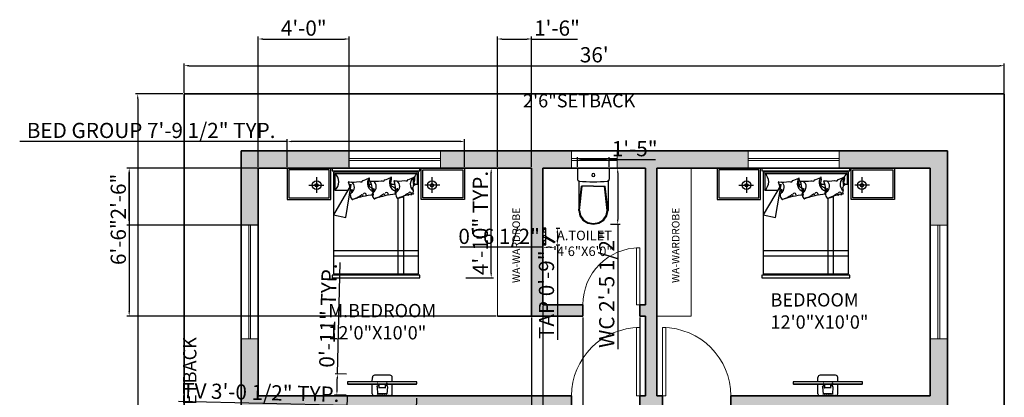
# Model space of a CAD drawing. Units: inches. Extents: x 4732 to 5926, y 2665 to 3255.
# Tile 6 of 8: x 4732 to 5250, y 3056 to 3255. Entities that reach past the tile are written whole.
import ezdxf

# ---------------------------------------------------------------- set-up
doc = ezdxf.new("R2010")
doc.units = ezdxf.units.IN
for name, color, linetype, lineweight in [('A-ANNO-DIMS', 2, 'Continuous', 18), ('A-ANNO-TEXT', 7, 'Continuous', 18), ('A-AREA-IDEN', 7, 'Continuous', 18), ('A-DOOR', 3, 'Continuous', 18), ('A-EQPM', 8, 'Continuous', 18), ('A-FLOR-CASE', 7, 'Continuous', 18), ('A-GLAZ', 4, 'Continuous', 18), ('A-WALL', 7, 'Continuous', 35), ('A-WALL-PATT', 8, 'Continuous', 13), ('C-PROP', 7, 'Continuous', 35), ('NOI THAT', 42, 'Continuous', 18), ('Сантехника', 7, 'Continuous', 18)]:
    doc.layers.add(name, color=color, linetype=linetype, lineweight=lineweight)
for name, color, linetype in [('FUR', 42, 'Continuous'), ('HA', 9, 'Continuous'), ('HID', 11, 'Continuous'), ('SAN', 5, 'Continuous'), ('SANTEH', 7, 'Continuous'), ('window', 130, 'Continuous')]:
    doc.layers.add(name, color=color, linetype=linetype)
doc.styles.get("Standard").update_dxf_attribs({"font": 'arial.ttf'})
doc.dimstyles.new('ISO-25', dxfattribs={"dimtxt": 8, "dimasz": 2.5, "dimexe": 1.25, "dimexo": 0.625, "dimtad": 1, "dimdec": 1, "dimlunit": 3, "dimtxsty": 'Standard', "dimcen": 2.5, "dimadec": 0, "dimazin": 0, "dimtfac": 1, "dimtdec": 1, "dimtmove": 0, "dimatfit": 3, "dimfxl": 1, "dimarcsym": 0})

# ---------------------------------------------------------------- blocks, each defined once
blk = doc.blocks.new('*D1')
at = {"layer": 'A-ANNO-DIMS', "color": 0, "lineweight": -2, "transparency": 16777216}
for p, q in [((4818.38, 3216.56), (4818.38, 3232.07)), ((5250.38, 3216.56), (5250.38, 3232.07)), ((4820.88, 3230.82), (5247.88, 3230.82))]:
    blk.add_line(p, q, dxfattribs=at)
at = {"layer": 'A-ANNO-DIMS', "color": 0, "transparency": 16777216}
for points in [[(4820.88, 3231.24), (4820.88, 3230.41), (4818.38, 3230.82)], [(5247.88, 3231.24), (5247.88, 3230.41), (5250.38, 3230.82)]]:
    blk.add_solid(points, dxfattribs=at)
at = {"layer": 'Defpoints', "color": 0, "transparency": 16777216}
for p in [(5250.38, 3230.82), (4818.38, 3215.93), (5250.38, 3215.93)]:
    blk.add_point(p, dxfattribs=at)
at = {"layer": 'A-ANNO-DIMS', "color": 0, "transparency": 16777216, "insert": (5034.38, 3235.54), "char_height": 8, "attachment_point": 5}
blk.add_mtext("36'", dxfattribs=at)
blk = doc.blocks.new('A$C73A16738')
at = {"layer": 'FUR'}
for p, q in [((1.15, 2.389), (1.1, 2.164)), ((1.7, 2.064), (1.15, 2.389)), ((1.6, 2.364), (1.6, 2.123)), ((1.9, 2.364), (1.6, 2.364)), ((1.9, 2.364), (1.9, 0.864)), ((1.1, 2.164), (1.7, 2.064)), ((1.7, 2.099), (1.7, 2.064)), ((1.7, 1.695), (1.7, 1.735)), ((1.7, 1.268), (1.7, 1.33)), ((1.7, 0.839), (1.7, 0.904)), ((1.9, 0.864), (1.7, 0.864))]:
    blk.add_line(p, q, dxfattribs=at)
for points in [[(1.428, 2.439), (2, 2.439), (2, 3.229), (1.428, 3.229)], [(1.458, 2.469), (1.97, 2.469), (1.97, 3.199), (1.458, 3.199)], [(0, 2.414), (0, 0.814), (0.05, 0.814), (0.05, 2.414)], [(0.075, 0.839), (1.925, 0.839), (1.925, 2.389), (0.075, 2.389)], [(1.95, 2.414), (1.95, 0.814), (2, 0.814), (2, 2.414)], [(1.428, 0.789), (2, 0.789), (2, 0), (1.428, 0)], [(1.458, 0.759), (1.97, 0.759), (1.97, 0.03), (1.458, 0.03)]]:
    blk.add_lwpolyline(points, close=True, dxfattribs=at)
for centre, start, end in [((1.75, 2.481), 217.7826, 322.2174), ((1.75, 0.748), 37.7826, 105.2747)]:
    blk.add_arc(centre, 0.19, start, end, dxfattribs=at)
at = {"layer": 'HA'}
for p, q in [((0.4, 2.389), (0.4, 0.839)), ((0.5, 2.389), (0.5, 0.839)), ((1.446, 1.214), (0.075, 1.214)), ((1.477, 1.114), (0.075, 1.114))]:
    blk.add_line(p, q, dxfattribs=at)
at = {"layer": 'HID'}
for centre, radius, start, end in [((1.442, 2.042), 0.0144, 131.666, 199.4465), ((0.016, 1.539), 1.498, 4.5852, 19.4465), ((0.016, 1.539), 1.498, 16.386, 19.4465), ((1.51, 1.965), 0.117, 87.3377, 131.666), ((1.515, 2.068), 0.0144, 51.6071, 87.3377), ((1.617, 2.197), 0.15, 231.6071, 269.7845), ((1.65, 2.128), 0.12, 212.7628, 323.8922), ((1.592, 2.074), 0.0072, 92.7363, 208.2985), ((1.628, 2.093), 0.0475, 208.2985, 255.7891), ((1.569, 2.56), 0.48, 272.7363, 290.959), ((1.743, 2.106), 0.0072, 352.7248, 110.959), ((2.348, 2.029), 0.603, 172.7248, 190.2702), ((1.467, 1.966), 0.0144, 196.386, 223.7955), ((0.926, 1.551), 0.667, 29.049, 37.3823), ((1.51, 1.823), 0.0319, 112.7015, 147.1556), ((1.51, 1.821), 0.0305, 232.3565, 65.7762), ((1.503, 1.839), 0.0144, 102.6426, 112.7015), ((1.497, 1.868), 0.0144, 282.6426, 29.049), ((2.038, 1.868), 0.288, 169.4168, 179.3085), ((1.758, 1.872), 0.0072, 179.3085, 290.689), ((1.763, 1.858), 0.0072, 16.2196, 110.689), ((2.348, 2.029), 0.603, 196.2196, 208.2114), ((1.455, 1.642), 0.0144, 131.666, 199.4465), ((0.03, 1.139), 1.498, 4.5852, 19.4465), ((0.03, 1.139), 1.498, 16.386, 19.4465), ((1.524, 1.565), 0.117, 87.3377, 131.666), ((1.524, 1.653), 0.0144, 67.1663, 184.3422), ((1.529, 1.668), 0.0144, 51.6071, 87.3377), ((1.574, 1.774), 0.117, 247.1663, 295.7613), ((1.631, 1.797), 0.15, 231.6071, 269.7845), ((1.663, 1.728), 0.12, 212.7628, 323.8922), ((1.722, 1.609), 0.162, 53.8947, 162.3952), ((1.606, 1.674), 0.0072, 92.7363, 208.2985), ((1.642, 1.693), 0.0475, 208.2985, 255.7891), ((1.583, 2.161), 0.48, 272.7363, 290.959), ((2.854, 0.961), 1.418, 145.8329, 150.0245), ((3.143, 2.369), 1.611, 202.7018, 202.7206), ((1.683, 1.758), 0.0288, 232.662, 339.1573), ((1.686, 1.753), 0.0072, 38.8315, 145.8329), ((1.788, 1.924), 0.192, 239.9211, 277.124), ((0.088, 1.831), 1.611, 356.4982, 357.2888), ((1.757, 1.706), 0.0072, 352.7248, 110.959), ((2.362, 1.629), 0.603, 172.7248, 190.2702), ((1.811, 1.74), 0.0072, 277.124, 28.2114), ((1.811, 1.74), 0.0072, 277.124, 28.2114), ((1.48, 1.566), 0.0144, 196.386, 223.7955), ((0.94, 1.151), 0.667, 29.049, 37.3823), ((1.523, 1.423), 0.0319, 112.7015, 147.1556), ((1.523, 1.422), 0.0305, 232.3565, 65.7762), ((1.517, 1.44), 0.0144, 102.6426, 112.7015), ((1.51, 1.468), 0.0144, 282.6426, 29.049), ((2.052, 1.468), 0.288, 169.4168, 179.3085), ((1.771, 1.472), 0.0072, 179.3085, 290.689), ((1.776, 1.458), 0.0072, 16.2196, 110.689), ((2.362, 1.629), 0.603, 196.2196, 208.2114), ((1.529, 1.139), 0.117, 87.3377, 131.666), ((1.537, 1.254), 0.0144, 67.1663, 184.3422), ((1.533, 1.242), 0.0144, 51.6071, 87.3377), ((1.588, 1.374), 0.117, 247.1663, 295.7613), ((1.736, 1.209), 0.162, 53.8947, 162.3952), ((1.611, 1.248), 0.0072, 92.7363, 208.2985), ((1.588, 1.734), 0.48, 272.7363, 290.959), ((2.867, 0.561), 1.418, 145.8329, 150.0245), ((3.156, 1.97), 1.611, 202.7018, 202.7206), ((1.697, 1.359), 0.0288, 232.662, 339.1573), ((1.7, 1.353), 0.0072, 38.8315, 145.8329), ((1.802, 1.524), 0.192, 239.9211, 277.124), ((0.102, 1.431), 1.611, 356.4982, 357.2888), ((1.762, 1.28), 0.0072, 352.7248, 110.959), ((2.367, 1.203), 0.603, 172.7248, 190.2702), ((1.825, 1.34), 0.0072, 277.124, 28.2114), ((1.825, 1.34), 0.0072, 277.124, 28.2114), ((1.46, 1.216), 0.0144, 131.666, 199.4465), ((0.688, 0.841), 0.844, 6.224, 26.0326), ((0.034, 0.713), 1.498, 16.386, 19.4465), ((1.485, 1.14), 0.0144, 196.386, 223.7955), ((0.945, 0.725), 0.667, 29.049, 37.3823), ((1.635, 1.371), 0.15, 231.6071, 269.7845), ((1.668, 1.302), 0.12, 212.7628, 323.8922), ((1.646, 1.267), 0.0475, 208.2985, 255.7891), ((2.056, 1.042), 0.288, 169.4168, 179.3085), ((1.528, 0.997), 0.0319, 112.7015, 147.1556), ((1.528, 0.995), 0.0305, 232.3565, 65.7762), ((1.521, 1.013), 0.0144, 102.6426, 112.7015), ((1.515, 1.042), 0.0144, 282.6426, 29.049), ((1.542, 0.927), 0.0144, 67.1663, 184.3422), ((1.593, 1.048), 0.117, 247.1663, 295.7613), ((1.705, 0.84), 0.15, 29.3598, 142.4281), ((1.581, 0.528), 0.419, 73.7524, 81.4605), ((3.161, 1.543), 1.611, 202.7018, 202.7206), ((1.702, 0.932), 0.0288, 232.662, 339.1573), ((1.705, 0.927), 0.0072, 38.8315, 145.8329), ((0.106, 1.005), 1.611, 356.4982, 357.2888), ((1.806, 1.098), 0.192, 246.1093, 277.124), ((1.776, 1.046), 0.0072, 179.3085, 290.689), ((1.781, 1.032), 0.0072, 16.2196, 110.689), ((2.367, 1.203), 0.603, 196.2196, 208.2114), ((1.829, 0.914), 0.0072, 277.124, 28.2114), ((1.829, 0.914), 0.0072, 277.124, 28.2114)]:
    blk.add_arc(centre, radius, start, end, dxfattribs=at)
at = {"layer": 'SAN'}
for p, q in [((1.832, 2.695), (1.546, 2.695)), ((1.688, 2.835), (1.688, 2.566)), ((1.688, 0.454), (1.688, 0.723)), ((1.832, 0.594), (1.546, 0.594))]:
    blk.add_line(p, q, dxfattribs=at)
for centre, radius in [((1.688, 2.695), 0.08), ((1.688, 2.695), 0.03), ((1.688, 0.594), 0.08), ((1.688, 0.594), 0.03)]:
    blk.add_circle(centre, radius, dxfattribs=at)
blk = doc.blocks.new('*U19')
for p, q in [((0, 0), (0, -6)), ((30, 0), (30, -6))]:
    blk.add_line(p, q)
blk.add_lwpolyline([(0, 0), (0, 30), (1.75, 30), (1.75, 0)], close=True)
blk.add_arc((0, 0), 30, 0, 90)
blk = doc.blocks.new('*U20')
for p, q in [((0, 0), (0, -6)), ((36, 0), (36, -6))]:
    blk.add_line(p, q)
blk.add_lwpolyline([(0, 0), (0, 36), (1.75, 36), (1.75, 0)], close=True)
blk.add_arc((0, 0), 36, 0, 90)
blk = doc.blocks.new('WC 2 Symb_109')
at = {"layer": 'SANTEH'}
for p, q in [((0, 0), (0, 380)), ((0, 380), (132, 380)), ((154, 365), (507, 365)), ((506, 365), (216, 331)), ((506, 356), (216, 322)), ((216, 190), (216, 331)), ((216, 190), (216, 49)), ((154, 15), (507, 15)), ((506, 24), (216, 58)), ((506, 15), (216, 49)), ((0, 0), (132, 0))]:
    blk.add_line(p, q, dxfattribs=at)
for points in [[(155, 360), (154, 364), (152, 368), (150, 371), (147, 374), (144, 377), (140, 379), (137, 380), (132, 380)], [(155, 20), (159, 62), (161, 105), (163, 147), (164, 190), (163, 233), (161, 275), (159, 318), (155, 360)], [(506, 24), (565, 37), (616, 73), (649, 126), (661, 190), (649, 254), (616, 307), (565, 343), (506, 356)], [(507, 15), (569, 28), (622, 66), (658, 123), (670, 190), (658, 257), (622, 314), (569, 352), (507, 365)], [(132, 0), (136, 0), (140, 1), (144, 3), (147, 6), (150, 9), (152, 12), (154, 16), (155, 20)]]:
    blk.add_lwpolyline(points, dxfattribs=at)
blk.add_lwpolyline([(84, 208), (70, 203), (65, 190), (70, 177), (84, 172), (97, 177), (102, 190), (97, 203)], close=True, dxfattribs=at)
blk = doc.blocks.new('Faucet - kit sink top')
at = {"layer": 'SANTEH'}
for p, q in [((-5.5, -0.75), (-5.5, -1.25)), ((-4.94278, -0.75), (-5.5, -0.75)), ((-5.5, -1.25), (-4.94278, -1.25)), ((-0.14775, -1.7441), (3.56698, -8.1782)), ((4.43301, -7.6782), (0.71828, -1.2441)), ((4.94278, -0.75), (5.5, -0.75)), ((5.5, -1.25), (4.94278, -1.25)), ((5.5, -0.75), (5.5, -1.25))]:
    blk.add_line(p, q, dxfattribs=at)
blk.add_lwpolyline([(-0.00587, -2), (-6, -2), (-6, 0), (6, 0), (6, -2), (1.15195, -2)], dxfattribs=at)
for centre, radius in [((-4, -1), 1), ((4, -1), 1), ((0, -1), 0.75)]:
    blk.add_circle(centre, radius, dxfattribs=at)
blk.add_arc((4, -7.9282), 0.5, 210, 30, dxfattribs=at)
blk = doc.blocks.new('TV')
at = {"color": 0}
for p, q in [((3967.27, 1784.85), (3967.05, 1784.65)), ((3967.76, 1763.68), (3967.54, 1763.86))]:
    blk.add_line(p, q, dxfattribs=at)
at = {"layer": 'window'}
for p, q in [((3967.54, 1763.86), (3967.05, 1784.65)), ((3966.53, 1775.82), (3964.33, 1775.61)), ((3964.34, 1775.34), (3964.45, 1775.34)), ((3964.34, 1775.31), (3964.43, 1775.32)), ((3964.41, 1777.23), (3967.22, 1777.3)), ((3966.14, 1775.2), (3967.01, 1775.22)), ((3966.14, 1775.18), (3967.27, 1775.2)), ((3966.14, 1775.18), (3966.14, 1775.2)), ((3966.3, 1773.29), (3966.26, 1775.18)), ((3968.01, 1777.32), (3969.36, 1777.35)), ((3964.39, 1773.06), (3964.48, 1773.06)), ((3964.39, 1773.04), (3964.5, 1773.04)), ((3966.61, 1772.66), (3964.4, 1772.77)), ((3966.19, 1773.28), (3967.31, 1773.31)), ((3966.19, 1773.26), (3967.05, 1773.28)), ((3966.19, 1773.26), (3966.19, 1773.28)), ((3964.55, 1771.15), (3967.36, 1771.22)), ((3968.15, 1771.24), (3969.5, 1771.27))]:
    blk.add_line(p, q, dxfattribs=at)
for points in [[(3968.33, 1763.69), (3967.83, 1784.86), (3967.27, 1784.85), (3967.76, 1763.68), (3968.33, 1763.69)], [(3963.86, 1771.81), (3963.75, 1776.54)], [(3964.4, 1772.77), (3964.33, 1775.61)], [(3964.48, 1773.06), (3964.43, 1775.32)], [(3964.5, 1773.04), (3964.45, 1775.34)], [(3970.16, 1771.96), (3970.05, 1776.69)]]:
    blk.add_lwpolyline(points, dxfattribs=at)
for points in [[(3966.53, 1775.82, -0.263666), (3966.93, 1775.69), (3967, 1775.57), (3967.01, 1775.22)], [(3966.61, 1772.66, 0.263666), (3967, 1772.81), (3967.06, 1772.93), (3967.05, 1773.28)]]:
    blk.add_lwpolyline(points, format="xyb", dxfattribs=at)
for centre, radius in [((3963.91, 1775.73), 0.0679), ((3963.93, 1775.17), 0.0679), ((3963.94, 1774.6), 0.0679), ((3967.77, 1775.68), 0.0451), ((3963.95, 1774.04), 0.0679), ((3963.97, 1773.48), 0.0679), ((3963.98, 1772.92), 0.0679), ((3963.99, 1772.35), 0.0679), ((3964.01, 1771.79), 0.0679), ((3967.83, 1772.86), 0.0451)]:
    blk.add_circle(centre, radius, dxfattribs=at)
for centre, start, end in [((3964.42, 1776.56), 91.3414, 181.3414), ((3969.38, 1776.67), 1.3414, 91.3414), ((3964.53, 1771.83), 181.3414, 271.3414), ((3969.49, 1771.94), 271.3414, 1.3414)]:
    blk.add_arc(centre, 0.676, start, end, dxfattribs=at)
blk = doc.blocks.new('*D28')
at = {"layer": 'A-ANNO-DIMS', "color": 0, "lineweight": -2, "transparency": 16777216}
for p, q in [((4817.76, 3215.93), (4792.67, 3215.93)), ((4793.92, 3213.43), (4793.92, 2738.43)), ((4817.76, 2735.93), (4792.67, 2735.93))]:
    blk.add_line(p, q, dxfattribs=at)
at = {"layer": 'A-ANNO-DIMS', "color": 0, "transparency": 16777216}
for points in [[(4793.5, 3213.43), (4794.33, 3213.43), (4793.92, 3215.93)], [(4793.5, 2738.43), (4794.33, 2738.43), (4793.92, 2735.93)]]:
    blk.add_solid(points, dxfattribs=at)
at = {"layer": 'Defpoints', "color": 0, "transparency": 16777216}
for p in [(4818.38, 3215.93), (4793.92, 2735.93), (4818.38, 2735.93)]:
    blk.add_point(p, dxfattribs=at)
at = {"layer": 'A-ANNO-DIMS', "color": 0, "transparency": 16777216, "insert": (4789.21, 2975.93), "char_height": 8, "attachment_point": 5, "rotation": 90}
blk.add_mtext("40'", dxfattribs=at)
blk = doc.blocks.new('GLAZ-UNIT-48IN')
for p, q in [((0, 1), (48, 1)), ((0, 0), (48, 0))]:
    blk.add_line(p, q)
blk = doc.blocks.new('GLAZ-UNIT-60IN')
for p, q in [((0, 0), (0, 60)), ((1, 0), (1, 60))]:
    blk.add_line(p, q)
blk = doc.blocks.new('GLAZ-UNIT-24IN')
for p, q in [((0, 1), (24, 1)), ((0, 0), (24, 0))]:
    blk.add_line(p, q)
blk = doc.blocks.new('*D74')
at = {"layer": 'A-ANNO-DIMS', "color": 0, "lineweight": -2, "transparency": 16777216}
for p, q in [((4872.72, 3190.94), (4731.74, 3190.94)), ((4872.72, 3177.56), (4872.72, 3192.19)), ((4963.6, 3190.94), (4875.22, 3190.94)), ((4966.1, 3177.56), (4966.1, 3192.19))]:
    blk.add_line(p, q, dxfattribs=at)
at = {"layer": 'A-ANNO-DIMS', "color": 0, "transparency": 16777216}
for points in [[(4875.22, 3191.36), (4875.22, 3190.52), (4872.72, 3190.94)], [(4963.6, 3191.36), (4963.6, 3190.52), (4966.1, 3190.94)]]:
    blk.add_solid(points, dxfattribs=at)
at = {"layer": 'Defpoints', "color": 0, "transparency": 16777216}
for p in [(4872.72, 3190.94), (4872.72, 3176.93), (4966.1, 3176.93)]:
    blk.add_point(p, dxfattribs=at)
at = {"layer": 'A-ANNO-DIMS', "color": 0, "transparency": 16777216, "insert": (4800.98, 3195.7), "char_height": 8, "attachment_point": 5, "rotation": 360}
blk.add_mtext('BED GROUP 7\'-9 1/2" TYP.', dxfattribs=at)
blk = doc.blocks.new('*D75')
at = {"layer": 'A-ANNO-DIMS', "color": 0, "lineweight": -2, "transparency": 16777216}
for p, q in [((4966.72, 3176.93), (4981.35, 3176.93)), ((4980.1, 3121.59), (4980.1, 3174.43)), ((4966.72, 3119.09), (4981.35, 3119.09))]:
    blk.add_line(p, q, dxfattribs=at)
at = {"layer": 'A-ANNO-DIMS', "color": 0, "transparency": 16777216}
for points in [[(4979.69, 3174.43), (4980.52, 3174.43), (4980.1, 3176.93)], [(4979.69, 3121.59), (4980.52, 3121.59), (4980.1, 3119.09)]]:
    blk.add_solid(points, dxfattribs=at)
at = {"layer": 'Defpoints', "color": 0, "transparency": 16777216}
for p in [(4966.1, 3176.93), (4980.1, 3176.93), (4966.1, 3119.09)]:
    blk.add_point(p, dxfattribs=at)
at = {"layer": 'A-ANNO-DIMS', "color": 0, "transparency": 16777216, "insert": (4975.4, 3148.01), "char_height": 8, "attachment_point": 5, "rotation": 90}
blk.add_mtext('4\'-10" TYP.', dxfattribs=at)
blk = doc.blocks.new('*D82')
at = {"layer": 'A-ANNO-DIMS', "color": 0, "lineweight": -2, "transparency": 16777216}
for p, q in [((4904.29, 3056.7), (4904.13, 3050.59)), ((4940.81, 3055.77), (4940.65, 3049.66)), ((4904.16, 3051.84), (4815.45, 3054.1)), ((4938.19, 3050.98), (4906.66, 3051.78))]:
    blk.add_line(p, q, dxfattribs=at)
at = {"layer": 'A-ANNO-DIMS', "color": 0, "transparency": 16777216}
for points in [[(4906.67, 3052.2), (4906.65, 3051.36), (4904.16, 3051.84)], [(4938.2, 3051.39), (4938.17, 3050.56), (4940.68, 3050.91)]]:
    blk.add_solid(points, dxfattribs=at)
at = {"layer": 'Defpoints', "color": 0, "transparency": 16777216}
for p in [(4904.3, 3057.32), (4940.82, 3056.39), (4904.16, 3051.84)]:
    blk.add_point(p, dxfattribs=at)
at = {"layer": 'A-ANNO-DIMS', "color": 0, "transparency": 16777216, "insert": (4858.68, 3057.76), "char_height": 8, "attachment_point": 5, "rotation": 358.5431}
blk.add_mtext('TV 3\'-0 1/2" TYP.', dxfattribs=at)
blk = doc.blocks.new('*D83')
at = {"layer": 'A-ANNO-DIMS', "color": 0, "lineweight": -2, "transparency": 16777216}
for p, q in [((4899.11, 3068.54), (4900.6, 3127.25)), ((4903.96, 3068.41), (4897.86, 3068.57)), ((4898.89, 3059.96), (4899.04, 3066.04)), ((4903.68, 3057.34), (4897.58, 3057.49))]:
    blk.add_line(p, q, dxfattribs=at)
at = {"layer": 'A-ANNO-DIMS', "color": 0, "transparency": 16777216}
for points in [[(4898.63, 3066.05), (4899.46, 3066.03), (4899.11, 3068.54)], [(4898.47, 3059.97), (4899.3, 3059.95), (4898.82, 3057.46)]]:
    blk.add_solid(points, dxfattribs=at)
at = {"layer": 'Defpoints', "color": 0, "transparency": 16777216}
for p in [(4899.11, 3068.54), (4904.58, 3068.4), (4904.3, 3057.32)]:
    blk.add_point(p, dxfattribs=at)
at = {"layer": 'A-ANNO-DIMS', "color": 0, "transparency": 16777216, "insert": (4895.18, 3099.26), "char_height": 8, "attachment_point": 5, "rotation": 88.5431}
blk.add_mtext('0\'-11" TYP.', dxfattribs=at)
blk = doc.blocks.new('*D98')
at = {"layer": 'A-ANNO-DIMS', "color": 0, "lineweight": -2, "transparency": 16777216}
for p, q in [((5042.94, 3176.93), (5048, 3176.93)), ((5046.75, 3174.43), (5046.75, 3149.83)), ((5042.94, 3147.33), (5048, 3147.33)), ((5046.75, 3147.33), (5046.75, 3081.62))]:
    blk.add_line(p, q, dxfattribs=at)
at = {"layer": 'A-ANNO-DIMS', "color": 0, "transparency": 16777216}
for points in [[(5046.34, 3174.43), (5047.17, 3174.43), (5046.75, 3176.93)], [(5046.34, 3149.83), (5047.17, 3149.83), (5046.75, 3147.33)]]:
    blk.add_solid(points, dxfattribs=at)
at = {"layer": 'Defpoints', "color": 0, "transparency": 16777216}
for p in [(5042.31, 3176.93), (5042.31, 3147.33), (5046.75, 3147.33)]:
    blk.add_point(p, dxfattribs=at)
at = {"layer": 'A-ANNO-DIMS', "color": 0, "transparency": 16777216, "insert": (5041.99, 3113.22), "char_height": 8, "attachment_point": 5, "rotation": 90}
blk.add_mtext('WC 2\'-5 1/2"', dxfattribs=at)
blk = doc.blocks.new('*D99')
at = {"layer": 'A-ANNO-DIMS', "color": 0, "lineweight": -2, "transparency": 16777216}
for p, q in [((5025.52, 3177.56), (5025.52, 3182.62)), ((5028.02, 3181.37), (5039.81, 3181.37)), ((5042.31, 3177.56), (5042.31, 3182.62)), ((5042.31, 3181.37), (5066.57, 3181.37))]:
    blk.add_line(p, q, dxfattribs=at)
at = {"layer": 'A-ANNO-DIMS', "color": 0, "transparency": 16777216}
for points in [[(5028.02, 3181.79), (5028.02, 3180.96), (5025.52, 3181.37)], [(5039.81, 3181.79), (5039.81, 3180.96), (5042.31, 3181.37)]]:
    blk.add_solid(points, dxfattribs=at)
at = {"layer": 'Defpoints', "color": 0, "transparency": 16777216}
for p in [(5042.31, 3181.37), (5025.52, 3176.93), (5042.31, 3176.93)]:
    blk.add_point(p, dxfattribs=at)
at = {"layer": 'A-ANNO-DIMS', "color": 0, "transparency": 16777216, "insert": (5055.69, 3186.08), "char_height": 8, "attachment_point": 5}
blk.add_mtext('1\'-5"', dxfattribs=at)
blk = doc.blocks.new('*D100')
at = {"layer": 'A-ANNO-DIMS', "color": 0, "lineweight": -2, "transparency": 16777216}
for p, q in [((5014.26, 3145.35), (5016.21, 3145.35)), ((5014.96, 3142.85), (5014.96, 3139.02)), ((5014.26, 3136.52), (5016.21, 3136.52)), ((5014.96, 3136.52), (5014.96, 3086.46))]:
    blk.add_line(p, q, dxfattribs=at)
at = {"layer": 'A-ANNO-DIMS', "color": 0, "transparency": 16777216}
for points in [[(5014.54, 3142.85), (5015.37, 3142.85), (5014.96, 3145.35)], [(5014.54, 3139.02), (5015.37, 3139.02), (5014.96, 3136.52)]]:
    blk.add_solid(points, dxfattribs=at)
at = {"layer": 'Defpoints', "color": 0, "transparency": 16777216}
for p in [(5013.63, 3145.35), (5013.63, 3136.52), (5014.96, 3136.52)]:
    blk.add_point(p, dxfattribs=at)
at = {"layer": 'A-ANNO-DIMS', "color": 0, "transparency": 16777216, "insert": (5010.25, 3110.24), "char_height": 8, "attachment_point": 5, "rotation": 90}
blk.add_mtext('TAP 0\'-9"', dxfattribs=at)
blk = doc.blocks.new('*D101')
at = {"layer": 'A-ANNO-DIMS', "color": 0, "lineweight": -2, "transparency": 16777216}
for p, q in [((5007.38, 3135.2), (4963.72, 3135.2)), ((5007.38, 3135.89), (5007.38, 3133.95)), ((5011.13, 3135.2), (5009.88, 3135.2)), ((5013.63, 3135.89), (5013.63, 3133.95))]:
    blk.add_line(p, q, dxfattribs=at)
at = {"layer": 'A-ANNO-DIMS', "color": 0, "transparency": 16777216}
for points in [[(5009.88, 3135.61), (5009.88, 3134.78), (5007.38, 3135.2)], [(5011.13, 3135.61), (5011.13, 3134.78), (5013.63, 3135.2)]]:
    blk.add_solid(points, dxfattribs=at)
at = {"layer": 'Defpoints', "color": 0, "transparency": 16777216}
for p in [(5007.38, 3136.52), (5007.38, 3135.2), (5013.63, 3136.52)]:
    blk.add_point(p, dxfattribs=at)
at = {"layer": 'A-ANNO-DIMS', "color": 0, "transparency": 16777216, "insert": (4984.3, 3139.96), "char_height": 8, "attachment_point": 5}
blk.add_mtext('0\'-6 1/2"', dxfattribs=at)
blk = doc.blocks.new('*D107')
at = {"layer": 'A-ANNO-DIMS', "color": 0, "lineweight": -2, "transparency": 16777216}
for p, q in [((5028.38, 3098.31), (5028.38, 2665.12)), ((5058.38, 3098.31), (5058.38, 2665.12)), ((5030.88, 2666.37), (5055.88, 2666.37))]:
    blk.add_line(p, q, dxfattribs=at)
at = {"layer": 'A-ANNO-DIMS', "color": 0, "transparency": 16777216}
for points in [[(5030.88, 2666.79), (5030.88, 2665.96), (5028.38, 2666.37)], [(5055.88, 2666.79), (5055.88, 2665.96), (5058.38, 2666.37)]]:
    blk.add_solid(points, dxfattribs=at)
at = {"layer": 'Defpoints', "color": 0, "transparency": 16777216}
for p in [(5028.38, 3098.93), (5058.38, 3098.93), (5058.38, 2666.37)]:
    blk.add_point(p, dxfattribs=at)
at = {"layer": 'A-ANNO-DIMS', "color": 0, "transparency": 16777216, "insert": (5043.38, 2671.08), "char_height": 8, "attachment_point": 5}
blk.add_mtext('2\'-6"', dxfattribs=at)
blk = doc.blocks.new('*D108')
at = {"layer": 'A-ANNO-DIMS', "color": 0, "lineweight": -2, "transparency": 16777216}
for p, q in [((4983.38, 3177.56), (4983.38, 3246.13)), ((4985.88, 3244.88), (4998.88, 3244.88)), ((5001.38, 3177.56), (5001.38, 3246.13)), ((5001.38, 3244.88), (5025.64, 3244.88))]:
    blk.add_line(p, q, dxfattribs=at)
at = {"layer": 'A-ANNO-DIMS', "color": 0, "transparency": 16777216}
for points in [[(4985.88, 3245.3), (4985.88, 3244.47), (4983.38, 3244.88)], [(4998.88, 3245.3), (4998.88, 3244.47), (5001.38, 3244.88)]]:
    blk.add_solid(points, dxfattribs=at)
at = {"layer": 'Defpoints', "color": 0, "transparency": 16777216}
for p in [(5001.38, 3244.88), (4983.38, 3176.93), (5001.38, 3176.93)]:
    blk.add_point(p, dxfattribs=at)
at = {"layer": 'A-ANNO-DIMS', "color": 0, "transparency": 16777216, "insert": (5014.76, 3249.59), "char_height": 8, "attachment_point": 5}
blk.add_mtext('1\'-6"', dxfattribs=at)
blk = doc.blocks.new('*D109')
at = {"layer": 'A-ANNO-DIMS', "color": 0, "lineweight": -2, "transparency": 16777216}
for p, q in [((4982.76, 3176.93), (4788.18, 3176.93)), ((4789.43, 3174.43), (4789.43, 3101.43)), ((4982.76, 3098.93), (4788.18, 3098.93))]:
    blk.add_line(p, q, dxfattribs=at)
at = {"layer": 'A-ANNO-DIMS', "color": 0, "transparency": 16777216}
for points in [[(4789.01, 3174.43), (4789.85, 3174.43), (4789.43, 3176.93)], [(4789.01, 3101.43), (4789.85, 3101.43), (4789.43, 3098.93)]]:
    blk.add_solid(points, dxfattribs=at)
at = {"layer": 'Defpoints', "color": 0, "transparency": 16777216}
for p in [(4983.38, 3176.93), (4789.43, 3098.93), (4983.38, 3098.93)]:
    blk.add_point(p, dxfattribs=at)
at = {"layer": 'A-ANNO-DIMS', "color": 0, "transparency": 16777216, "insert": (4784.72, 3137.93), "char_height": 8, "attachment_point": 5, "rotation": 90}
blk.add_mtext('6\'-6"', dxfattribs=at)
blk = doc.blocks.new('*D114')
at = {"layer": 'A-ANNO-DIMS', "color": 0, "lineweight": -2, "transparency": 16777216}
for p, q in [((5007.38, 3104.31), (5007.38, 2665.12)), ((5001.38, 3098.31), (5001.38, 2665.12)), ((4998.88, 2666.37), (4996.38, 2666.37)), ((5001.38, 2666.37), (5007.38, 2666.37)), ((5009.88, 2666.37), (5034.9, 2666.37))]:
    blk.add_line(p, q, dxfattribs=at)
at = {"layer": 'A-ANNO-DIMS', "color": 0, "transparency": 16777216}
for points in [[(4998.88, 2666.79), (4998.88, 2665.96), (5001.38, 2666.37)], [(5009.88, 2666.79), (5009.88, 2665.96), (5007.38, 2666.37)]]:
    blk.add_solid(points, dxfattribs=at)
at = {"layer": 'Defpoints', "color": 0, "transparency": 16777216}
for p in [(5007.38, 3104.93), (5001.38, 3098.93), (5007.38, 2666.37)]:
    blk.add_point(p, dxfattribs=at)
at = {"layer": 'A-ANNO-DIMS', "color": 0, "transparency": 16777216, "insert": (5023.64, 2671.08), "char_height": 8, "attachment_point": 5}
blk.add_mtext('0\'-6"', dxfattribs=at)
blk = doc.blocks.new('*D115')
at = {"layer": 'A-ANNO-DIMS', "color": 0, "lineweight": -2, "transparency": 16777216}
for p, q in [((4857.38, 3177.56), (4857.38, 3246.13)), ((4859.88, 3244.88), (4902.88, 3244.88)), ((4905.38, 3177.56), (4905.38, 3246.13))]:
    blk.add_line(p, q, dxfattribs=at)
at = {"layer": 'A-ANNO-DIMS', "color": 0, "transparency": 16777216}
for points in [[(4859.88, 3245.3), (4859.88, 3244.47), (4857.38, 3244.88)], [(4902.88, 3245.3), (4902.88, 3244.47), (4905.38, 3244.88)]]:
    blk.add_solid(points, dxfattribs=at)
at = {"layer": 'Defpoints', "color": 0, "transparency": 16777216}
for p in [(4905.38, 3244.88), (4857.38, 3176.93), (4905.38, 3176.93)]:
    blk.add_point(p, dxfattribs=at)
at = {"layer": 'A-ANNO-DIMS', "color": 0, "transparency": 16777216, "insert": (4881.38, 3249.59), "char_height": 8, "attachment_point": 5}
blk.add_mtext('4\'-0"', dxfattribs=at)
blk = doc.blocks.new('*D116')
at = {"layer": 'A-ANNO-DIMS', "color": 0, "lineweight": -2, "transparency": 16777216}
for p, q in [((4856.76, 3176.93), (4788.18, 3176.93)), ((4789.43, 3149.43), (4789.43, 3174.43)), ((4856.76, 3146.93), (4788.18, 3146.93))]:
    blk.add_line(p, q, dxfattribs=at)
at = {"layer": 'A-ANNO-DIMS', "color": 0, "transparency": 16777216}
for points in [[(4789.01, 3174.43), (4789.85, 3174.43), (4789.43, 3176.93)], [(4789.01, 3149.43), (4789.85, 3149.43), (4789.43, 3146.93)]]:
    blk.add_solid(points, dxfattribs=at)
at = {"layer": 'Defpoints', "color": 0, "transparency": 16777216}
for p in [(4789.43, 3176.93), (4857.38, 3176.93), (4857.38, 3146.93)]:
    blk.add_point(p, dxfattribs=at)
at = {"layer": 'A-ANNO-DIMS', "color": 0, "transparency": 16777216, "insert": (4784.72, 3161.93), "char_height": 8, "attachment_point": 5, "rotation": 90}
blk.add_mtext('2\'-6"', dxfattribs=at)

msp = doc.modelspace()

# ---------------------------------------------------------------- hatches: boundary and pattern name
at = {"layer": 'A-WALL-PATT'}
h = msp.add_hatch(color=256, dxfattribs=at)
h.dxf.hatch_style = 1
h.paths.add_polyline_path([(4905.38, 3185.93), (4848.38, 3185.93), (4848.38, 3146.93), (4857.38, 3146.93), (4857.38, 3176.93), (4905.38, 3176.93)])
h.paths.add_polyline_path([(5022.38, 3185.93), (4953.38, 3185.93), (4953.38, 3176.93), (4966.1, 3176.93), (5001.38, 3176.93), (5001.38, 3098.93), (5028.38, 3098.93), (5028.38, 3104.93), (5007.38, 3104.93), (5007.38, 3176.93), (5022.38, 3176.93)])
h.paths.add_polyline_path([(5115.38, 3185.93), (5046.38, 3185.93), (5046.38, 3176.93), (5061.38, 3176.93), (5061.38, 3104.93), (5058.38, 3104.93), (5058.38, 3098.93), (5067.38, 3098.93), (5067.38, 3176.93), (5115.38, 3176.93)])
h.paths.add_polyline_path([(5220.38, 3185.93), (5163.38, 3185.93), (5163.38, 3176.93), (5168.97, 3176.93), (5211.38, 3176.93), (5211.38, 3146.93), (5220.38, 3146.93)])
h.paths.add_polyline_path([(4857.38, 3086.93), (4848.38, 3086.93), (4848.38, 3026.93), (4857.38, 3026.93), (4857.38, 3050.93), (5001.38, 3050.93), (5001.38, 3008.93), (5007.38, 3008.93), (5007.38, 3050.93), (5022.38, 3050.93), (5022.38, 3056.93), (4857.38, 3056.93)])
h.paths.add_polyline_path([(4857.38, 2978.93), (4848.38, 2978.93), (4848.38, 2945.93), (4872.38, 2945.93), (4872.38, 2933.93), (4875.38, 2933.93), (4881.38, 2933.93), (4881.38, 2954.93), (4857.38, 2954.93)])
h.paths.add_polyline_path([(4881.38, 2903.93), (4875.38, 2903.93), (4872.38, 2903.93), (4872.38, 2897.93), (4881.38, 2897.93)])
h.paths.add_polyline_path([(4881.38, 2849.93), (4872.38, 2849.93), (4872.38, 2828.75), (4872.38, 2825.93), (4848.38, 2825.93), (4848.38, 2804.93), (4857.38, 2804.93), (4857.38, 2816.93), (4929.38, 2816.93), (4929.38, 2825.93), (4881.38, 2825.93)])
h.paths.add_polyline_path([(4975.38, 2744.93), (4857.38, 2744.93), (4857.38, 2756.93), (4848.38, 2756.93), (4848.38, 2735.93), (4975.38, 2735.93)])
h.paths.add_polyline_path([(5160.38, 2915.93), (5160.38, 2918.93), (5007.38, 2918.93), (5007.38, 2960.93), (5001.38, 2960.93), (5001.38, 2825.93), (4977.38, 2825.93), (4977.38, 2816.93), (5010.38, 2816.93), (5010.38, 2909.93), (5160.38, 2909.93)])
h.paths.add_polyline_path([(5220.38, 2948.93), (5211.38, 2948.93), (5211.38, 2918.93), (5208.38, 2918.93), (5208.38, 2909.93), (5220.38, 2909.93)])
h.paths.add_polyline_path([(5220.38, 3086.93), (5211.38, 3086.93), (5211.38, 3056.93), (5106.38, 3056.93), (5106.38, 3050.93), (5211.38, 3050.93), (5211.38, 3020.93), (5220.38, 3020.93)])
h.paths.add_polyline_path([(5067.38, 3098.93), (5061.38, 3098.93), (5061.38, 3056.93), (5058.38, 3056.93), (5058.38, 3050.93), (5061.38, 3050.93), (5070.38, 3050.93), (5070.38, 3056.93), (5067.38, 3056.93)])
h.paths.add_polyline_path([(4883.76, 2941.13), (4938.24, 2941.13), (4938.24, 2949.38), (4883.76, 2949.38)], flags=9)
h.paths.add_polyline_path([(4840.48, 3026.79), (4840.48, 3093.88), (4825.54, 3093.88), (4825.54, 3026.79)], flags=9)
h.paths.add_polyline_path([(5245.66, 2994.98), (5245.66, 3062.07), (5230.72, 3062.07), (5230.72, 2994.98)], flags=9)
h.paths.add_polyline_path([(4994.89, 3193.24), (5061.99, 3193.24), (5061.99, 3208.18), (4994.89, 3208.18)], flags=9)
h.paths.add_polyline_path([(5081.53, 3115.35), (5081.53, 3161.13), (5073.28, 3161.13), (5073.28, 3115.35)], flags=25)
h.paths.add_polyline_path([(4997.53, 3115.35), (4997.53, 3161.13), (4989.28, 3161.13), (4989.28, 3115.35)], flags=25)
h.paths.add_polyline_path([(5175.31, 2866.04), (5202.42, 2866.04), (5202.42, 2876.71), (5175.31, 2876.71)], flags=9)
h.paths.add_polyline_path([(4820.13, 2876.28), (4869.1, 2876.28), (4869.1, 2902.89), (4820.13, 2902.89)], flags=9)
h.paths.add_polyline_path([(5104.69, 2868.81), (5158.82, 2868.81), (5158.82, 2895.42), (5104.69, 2895.42)], flags=25)
h.paths.add_polyline_path([(5084.11, 2966.75), (5138.25, 2966.75), (5138.25, 2993.36), (5084.11, 2993.36)], flags=9)
h.paths.add_polyline_path([(4897.84, 3000.24), (4946.81, 3000.24), (4946.81, 3026.85), (4897.84, 3026.85)], flags=9)
h.paths.add_polyline_path([(5009.53, 3133.48), (5059.32, 3133.48), (5059.32, 3160.09), (5009.53, 3160.09)], flags=9)
h.paths.add_polyline_path([(5124.24, 3088.37), (5180.47, 3088.37), (5180.47, 3114.99), (5124.24, 3114.99)], flags=9)
h.paths.add_polyline_path([(4897.52, 3088.37), (4965.52, 3088.37), (4965.52, 3114.99), (4897.52, 3114.99)], flags=9)
h.paths.add_polyline_path([(4924.5, 2879.19), (4978.63, 2879.19), (4978.63, 2905.8), (4924.5, 2905.8)], flags=9)

# ---------------------------------------------------------------- linework, layer by layer
at = {"layer": 'A-FLOR-CASE'}
for p, q in [((4983.38, 3098.93), (4983.38, 3176.93)), ((5085.38, 3176.93), (5085.38, 3098.93)), ((5067.38, 3098.93), (5085.38, 3098.93))]:
    msp.add_line(p, q, dxfattribs=at)
at = {"layer": 'A-GLAZ'}
for p, q in [((4905.38, 3176.93), (4905.38, 3185.93)), ((4953.38, 3176.93), (4953.38, 3185.93)), ((5022.38, 3176.93), (5022.38, 3185.93)), ((5046.38, 3176.93), (5046.38, 3185.93)), ((5115.38, 3176.93), (5115.38, 3185.93)), ((5163.38, 3176.93), (5163.38, 3185.93)), ((4857.38, 3146.93), (4848.38, 3146.93)), ((5211.38, 3146.93), (5220.38, 3146.93)), ((4857.38, 3086.93), (4848.38, 3086.93)), ((5211.38, 3086.93), (5220.38, 3086.93))]:
    msp.add_line(p, q, dxfattribs=at)
at = {"layer": 'A-WALL'}
for p, q in [((4848.38, 3185.93), (5220.38, 3185.93)), ((4848.38, 2945.93), (4848.38, 3185.93)), ((5220.38, 3185.93), (5220.38, 2885.93)), ((4857.38, 3176.93), (5001.38, 3176.93)), ((4857.38, 3056.93), (4857.38, 3176.93)), ((5001.38, 3098.93), (5001.38, 3176.93)), ((5007.38, 3104.93), (5007.38, 3176.93)), ((5007.38, 3176.93), (5061.38, 3176.93)), ((5061.38, 3176.93), (5061.38, 3104.93)), ((5067.38, 3176.93), (5067.38, 3056.93)), ((5067.38, 3176.93), (5211.38, 3176.93)), ((5211.38, 3176.93), (5211.38, 3056.93)), ((5007.38, 3104.93), (5028.38, 3104.93)), ((5028.38, 3104.93), (5028.38, 3098.93)), ((5058.38, 3104.93), (5058.38, 3098.93)), ((5058.38, 3104.93), (5061.38, 3104.93)), ((4983.38, 3098.93), (5028.38, 3098.93)), ((5058.38, 3098.93), (5061.38, 3098.93)), ((5061.38, 3098.93), (5061.38, 3056.93)), ((4857.38, 3056.93), (5022.38, 3056.93)), ((5022.38, 3056.93), (5022.38, 3050.93)), ((5058.38, 3056.93), (5061.38, 3056.93)), ((5058.38, 3056.93), (5058.38, 3050.93)), ((5067.38, 3056.93), (5070.38, 3056.93)), ((5070.38, 3056.93), (5070.38, 3050.93)), ((5106.38, 3056.93), (5106.38, 3050.93)), ((5106.38, 3056.93), (5211.38, 3056.93))]:
    msp.add_line(p, q, dxfattribs=at)
at = {"layer": 'C-PROP'}
msp.add_lwpolyline([(4818.38, 3215.93), (5250.38, 3215.93), (5250.38, 2735.93), (4818.38, 2735.93)], close=True, dxfattribs=at)

# ---------------------------------------------------------------- block references
at = {"layer": 'A-DOOR', "xscale": -1}
for name, p in [('*U19', (5058.38, 3104.93)), ('*U20', (5058.38, 3056.93))]:
    msp.add_blockref(name, p, dxfattribs=at)
at = {"layer": 'A-DOOR'}
msp.add_blockref('*U20', (5070.38, 3056.93), dxfattribs=at)
at = {"layer": 'A-EQPM', "xscale": 1.724488909621177, "yscale": 1.724488909621177, "zscale": 1.724488909621177, "rotation": 88.54308451816136}
for p in [(7807.49, -3854.16), (8042.17, -3854.16)]:
    msp.add_blockref('TV', p, dxfattribs=at)
at = {"layer": 'A-GLAZ'}
for name, p in [('GLAZ-UNIT-48IN', (4905.38, 3180.93)), ('GLAZ-UNIT-24IN', (5022.38, 3180.93)), ('GLAZ-UNIT-48IN', (5115.38, 3180.93)), ('GLAZ-UNIT-60IN', (4852.38, 3086.93))]:
    msp.add_blockref(name, p, dxfattribs=at)
at = {"layer": 'A-GLAZ', "rotation": 180}
msp.add_blockref('GLAZ-UNIT-60IN', (5216.38, 3146.93), dxfattribs=at)
at = {"layer": 'NOI THAT', "xscale": 28.92215291203286, "yscale": 28.92215291203286, "zscale": 28.92215291203286, "rotation": 89.99999999852635}
for p in [(4966.1, 3119.09), (5192.53, 3119.09)]:
    msp.add_blockref('A$C73A16738', p, dxfattribs=at)
at = {"layer": 'Сантехника'}
for name, p, xscale, yscale, zscale, rotation in [('WC 2 Symb_109', (5025.52, 3176.93), 0.0441898926459964, 0.0441898926459964, 0.0441898926459964, 270), ('Faucet - kit sink top', (5007.38, 3140.93), -0.7356136897818673, 0.7356136897818673, 0.7356136897818673, 90)]:
    msp.add_blockref(name, p, dxfattribs=dict(at, xscale=xscale, yscale=yscale, zscale=zscale, rotation=rotation))

# ---------------------------------------------------------------- texts
at = {"layer": 'A-ANNO-TEXT', "insert": (4996.86, 3215.89), "char_height": 7, "attachment_point": 1}
msp.add_mtext_dynamic_manual_height_columns('{\\fTimes New Roman|b0|i0|c0|p18; 2\'6"SETBACK }', width=61.0557, gutter_width=12.5, heights=[0], dxfattribs=at)
at = {"layer": 'A-ANNO-TEXT', "attachment_point": 1, "rotation": 90}
for s, width, insert, char_height in [('WA-WARDROBE', 29.5334, (4991.27, 3116.42), 4), ('WA-WARDROBE', 29.5334, (5075.27, 3116.42), 4), ('{\\fTimes New Roman|b0|i0|c0|p18; 2\'6"SETBACK }', 61.0557, (4817.83, 3028.76), 7)]:
    msp.add_mtext_dynamic_manual_height_columns(s, width=width, gutter_width=12.5, heights=[0], dxfattribs=dict(at, insert=insert, char_height=char_height))
at = {"layer": 'A-AREA-IDEN', "attachment_point": 1}
for s, insert, char_height in [('{\\fTimes New Roman|b0|i0|c0|p18;A.TOILET\\P4\'6"X6\'0"}', (5014.72, 3143.95), 5), ('{\\fTimes New Roman|b0|i0|c0|p18;BEDROOM\\P12\'0"X10\'0"}', (5127.2, 3111.03), 7), ('{\\fTimes New Roman|b0|i0|c0|p18;M.BEDROOM\\P12\'0"X10\'0"}', (4894.3, 3105.37), 7)]:
    msp.add_mtext_dynamic_manual_height_columns(s, width=61.0557, gutter_width=12.5, heights=[0], dxfattribs=dict(at, insert=insert, char_height=char_height))

# ---------------------------------------------------------------- dimensions: what is measured, and where the dimension line sits
at = {"layer": 'A-ANNO-DIMS'}
for base, p1, p2, override, picture, middle in [((4905.38, 3244.88), (4857.38, 3176.93), (4905.38, 3176.93), {"dimdec": 1, "dimlfac": 1, "dimrnd": 0, "dimzin": 1, "dimdsep": 46, "dimlunit": 4, "dimfrac": 2}, '*D115', (4881.38, 3249.59)), ((5001.38, 3244.88), (4983.38, 3176.93), (5001.38, 3176.93), {"dimdec": 1, "dimlfac": 1, "dimrnd": 0, "dimzin": 1, "dimdsep": 46, "dimlunit": 4, "dimfrac": 2}, '*D108', (5014.76, 3249.59)), ((5250.38, 3230.82), (4818.38, 3215.93), (5250.38, 3215.93), {"dimclrd": 0, "dimclre": 0, "dimclrt": 0}, '*D1', (5034.38, 3235.54)), ((5042.31, 3181.37), (5025.52, 3176.93), (5042.31, 3176.93), {"dimdec": 1, "dimlfac": 1, "dimrnd": 0, "dimzin": 1, "dimdsep": 46, "dimlunit": 4, "dimfrac": 2}, '*D99', (5055.69, 3186.08)), ((5007.38, 2666.37), (5001.38, 3098.93), (5007.38, 3104.93), {"dimdec": 1, "dimlfac": 1, "dimrnd": 0, "dimzin": 1, "dimdsep": 46, "dimlunit": 4, "dimfrac": 2}, '*D114', (5023.64, 2671.08)), ((5058.38, 2666.37), (5028.38, 3098.93), (5058.38, 3098.93), {"dimdec": 1, "dimlfac": 1, "dimrnd": 0, "dimzin": 1, "dimdsep": 46, "dimlunit": 4, "dimfrac": 2}, '*D107', (5043.38, 2671.08))]:
    dim = msp.add_linear_dim(base=base, p1=p1, p2=p2, dimstyle='ISO-25', override=override, dxfattribs=at)
    dim.commit()
    dim.dimension.update_dxf_attribs({"geometry": picture, "text_midpoint": middle})
for base, p1, p2, angle, text, picture, middle in [((4872.72, 3190.94), (4966.1, 3176.93), (4872.72, 3176.93), 180, 'BED GROUP <> TYP.', '*D74', (4800.98, 3195.7)), ((4980.1, 3176.93), (4966.1, 3119.09), (4966.1, 3176.93), 90, '<> TYP.', '*D75', (4975.4, 3148.01)), ((5046.75, 3147.33), (5042.31, 3176.93), (5042.31, 3147.33), 270, 'WC <>', '*D98', (5041.99, 3113.22)), ((5014.96, 3136.52), (5013.63, 3145.35), (5013.63, 3136.52), 270, 'TAP <>', '*D100', (5010.25, 3110.24)), ((4899.11, 3068.54), (4904.3, 3057.32), (4904.58, 3068.4), 88.5431, '<> TYP.', '*D83', (4895.18, 3099.26)), ((4904.16, 3051.84), (4940.82, 3056.39), (4904.3, 3057.32), 178.5431, 'TV <> TYP.', '*D82', (4858.68, 3057.76))]:
    dim = msp.add_linear_dim(base=base, p1=p1, p2=p2, angle=angle, text=text, dimstyle='ISO-25', override={"dimdec": 1, "dimlfac": 1, "dimrnd": 0, "dimzin": 1, "dimdsep": 46, "dimlunit": 4, "dimfrac": 2}, dxfattribs=at)
    dim.commit()
    dim.dimension.update_dxf_attribs({"geometry": picture, "text_midpoint": middle})
for base, p1, p2, angle, override, picture, middle in [((4793.92, 2735.93), (4818.38, 3215.93), (4818.38, 2735.93), 90, {"dimclrd": 0, "dimclre": 0, "dimclrt": 0}, '*D28', (4789.21, 2975.93)), ((4789.43, 3098.93), (4983.38, 3176.93), (4983.38, 3098.93), 90, {"dimdec": 1, "dimlfac": 1, "dimrnd": 0, "dimzin": 1, "dimdsep": 46, "dimlunit": 4, "dimfrac": 2}, '*D109', (4784.72, 3137.93)), ((4789.43, 3176.93), (4857.38, 3146.93), (4857.38, 3176.93), 90, {"dimdec": 1, "dimlfac": 1, "dimrnd": 0, "dimzin": 1, "dimdsep": 46, "dimlunit": 4, "dimfrac": 2}, '*D116', (4784.72, 3161.93)), ((5007.3815, 3135.1955), (5013.6337, 3136.5196), (5007.3815, 3136.5196), 180, {"dimdec": 1, "dimlfac": 1, "dimrnd": 0, "dimzin": 1, "dimdsep": 46, "dimlunit": 4, "dimfrac": 2}, '*D101', (4984.3029, 3139.957))]:
    dim = msp.add_linear_dim(base=base, p1=p1, p2=p2, angle=angle, dimstyle='ISO-25', override=override, dxfattribs=at)
    dim.commit()
    dim.dimension.update_dxf_attribs({"geometry": picture, "text_midpoint": middle})

doc.saveas('drawing.dxf')
